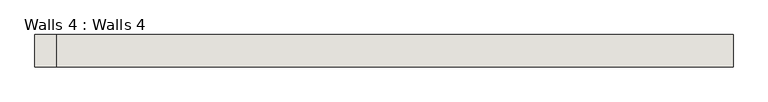
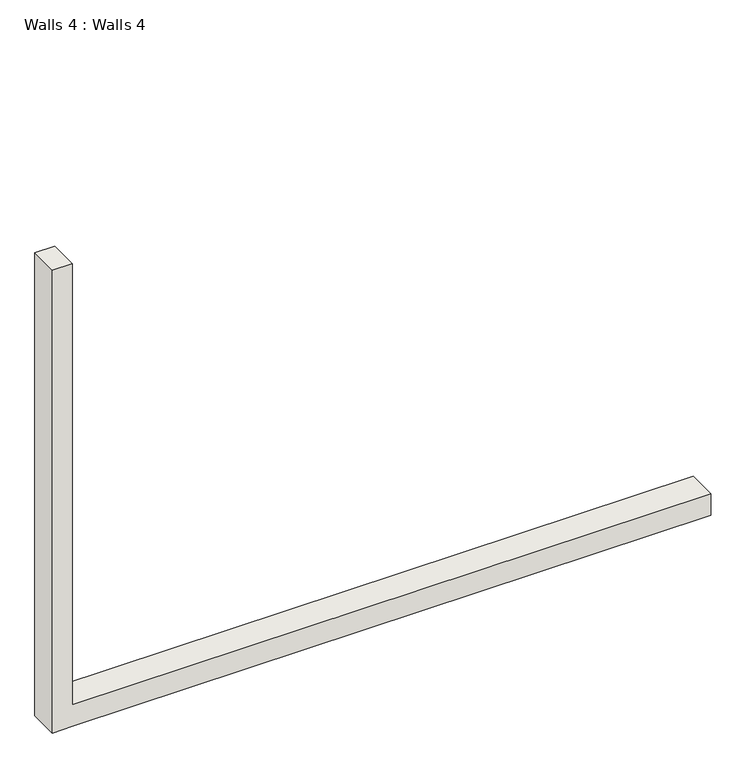
"""IFC4 building model written with IfcOpenShell, lengths in millimetres: wall geometry, Walls 4 : Walls 4."""

from ifc_helpers import new_model, si_unit, frame, origin, place, context, project, spatial, polyline, outline, extrude, source, transform, mapped, element, save


def walls_4_walls_4_0e46dea8(model_context):
    return source(origin(), model_context, "Body", "SweptSolid", [
        extrude(outline(polyline([(2648.0, -12513.0996792), (2648.0, -12313.0996792), (2648.0, -5912.2996792), (2876.6, -5912.2996792), (2876.6, -12313.0996792), (7554.2207413, -12313.0996792), (7554.2207413, -12513.0996792), (2648.0, -12513.0996792)])), frame((0.0, -7794.8501996, 0.0), z_axis=(0.0, 1.0, 0.0), x_axis=(0.0, 0.0, 1.0)), (0.0, 0.0, 1.0), 304.8),
    ])


if __name__ == "__main__":
    model = new_model("IFC4")
    model_context = context("Model", 3, world=origin())
    ifc_project = project(units=[si_unit("LENGTHUNIT", "METRE", prefix="MILLI")], contexts=[model_context])
    site = spatial("IfcSite", under=ifc_project)
    building = spatial("IfcBuilding", under=site)
    placement = place(None, origin())
    walls_4_walls_4_shape = walls_4_walls_4_0e46dea8(model_context)
    element("IfcWall", 1, ObjectType="Walls 4 : Walls 4", at=placement, inside=building, context=model_context, shape_type="MappedRepresentation", body=[
        mapped(walls_4_walls_4_shape, transform((0.0, 0.0, 0.0), x_axis=(1.0, 0.0, 0.0), y_axis=(0.0, 1.0, 0.0), z_axis=(0.0, 0.0, 1.0))),
    ])
    save(model, "model.ifc")

# Revit data of these elements
# Element 1 (IfcWall, "Walls 4 : Walls 4")
#   Materials on its faces: "Default Wall"
# Materials
#   "Default Wall": colour RGB 80 80 80, transparency 0
